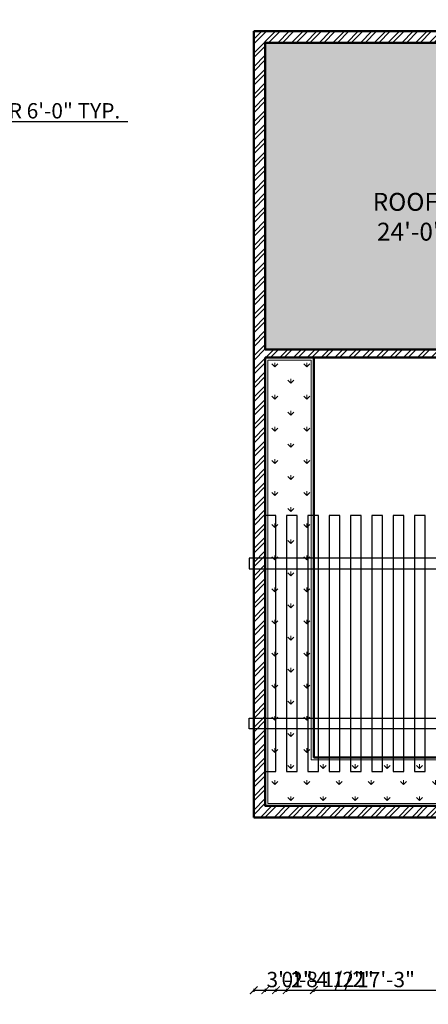
# Model space of a CAD drawing. Units: inches. Extents: x 261 to 2725, y 291 to 1454.
# Tile 26 of 35: x 1824 to 2144, y 293 to 1064. Entities that reach past the tile are written whole.
import ezdxf

# ---------------------------------------------------------------- set-up
doc = ezdxf.new("R2010")
doc.units = ezdxf.units.IN
for name, color, linetype, lineweight in [('A-ANNO-DIMS', 136, 'Continuous', 18), ('A-AREA-IDEN', 18, 'Continuous', 18), ('A-PLNT', 3, 'Continuous', 18), ('A-PLNT-PATT', 3, 'Continuous', 13), ('A-ROOF-PRGL', 25, 'Continuous', 25), ('A-WALL', 222, 'Continuous', 50), ('A-WALL-PATT', 243, 'Continuous', 13)]:
    doc.layers.add(name, color=color, linetype=linetype, lineweight=lineweight)
doc.styles.get("Standard").update_dxf_attribs({"font": 'arial.ttf'})
doc.dimstyles.new('ISO-25', dxfattribs={"dimtxt": 12, "dimasz": 6, "dimexe": 1.25, "dimexo": 0.625, "dimtad": 1, "dimdec": 0, "dimlunit": 3, "dimtxsty": 'Standard', "dimblk": 'ARCHTICK', "dimcen": 2.5, "dimadec": 0, "dimazin": 0, "dimtfac": 1, "dimtdec": 0, "dimtmove": 0, "dimatfit": 3, "dimfxl": 1, "dimfxlon": 1, "dimarcsym": 0})

# ---------------------------------------------------------------- blocks, each defined once
blk = doc.blocks.new('_ArchTick')
at = {"color": 0, "linetype": 'ByBlock', "const_width": 0.15}
blk.add_lwpolyline([(-0.5, -0.5), (0.5, 0.5)], dxfattribs=at)
blk = doc.blocks.new('*D63')
at = {"layer": 'A-ANNO-DIMS', "color": 0, "lineweight": -2, "ltscale": 0.07, "transparency": 16777216}
for p, q in [((1630.08, 983.27), (1630.08, 985.52)), ((1630.08, 984.27), (1702.08, 984.27)), ((1702.08, 983.27), (1702.08, 985.52)), ((1702.08, 984.27), (1909.1, 984.27))]:
    blk.add_line(p, q, dxfattribs=at)
at = {"layer": 'Defpoints', "color": 0, "ltscale": 0.07, "transparency": 16777216}
for p in [(1702.08, 984.27), (1630.08, 973.47), (1702.08, 973.47)]:
    blk.add_point(p, dxfattribs=at)
at = {"layer": 'A-ANNO-DIMS', "color": 0, "lineweight": -2, "ltscale": 0.07, "transparency": 16777216, "xscale": 6, "yscale": 6, "zscale": 6, "rotation": 180}
blk.add_blockref('_ArchTick', (1630.08, 984.27), dxfattribs=at)
at = {"layer": 'A-ANNO-DIMS', "color": 0, "lineweight": -2, "ltscale": 0.07, "transparency": 16777216, "xscale": 6, "yscale": 6, "zscale": 6}
blk.add_blockref('_ArchTick', (1702.08, 984.27), dxfattribs=at)
at = {"layer": 'A-ANNO-DIMS', "color": 0, "ltscale": 0.07, "transparency": 16777216, "insert": (1808.59, 991.1), "char_height": 12, "attachment_point": 5}
blk.add_mtext('SLIDING DOOR 6\'-0" TYP.', dxfattribs=at)
blk = doc.blocks.new('*D82')
at = {"layer": 'A-ANNO-DIMS', "color": 0, "lineweight": -2, "ltscale": 0.07, "transparency": 16777216}
for p, q in [((2600.96, 679.47), (2603.21, 679.47)), ((2601.96, 517.47), (2601.96, 679.47)), ((2600.96, 517.47), (2603.21, 517.47))]:
    blk.add_line(p, q, dxfattribs=at)
at = {"layer": 'Defpoints', "color": 0, "ltscale": 0.07, "transparency": 16777216}
for p in [(946.45, 679.47), (2601.96, 679.47), (946.45, 517.47)]:
    blk.add_point(p, dxfattribs=at)
at = {"layer": 'A-ANNO-DIMS', "color": 0, "lineweight": -2, "ltscale": 0.07, "transparency": 16777216, "xscale": 6, "yscale": 6, "zscale": 6}
for p, rotation in [((2601.96, 679.47), 90), ((2601.96, 517.47), 270)]:
    blk.add_blockref('_ArchTick', p, dxfattribs=dict(at, rotation=rotation))
at = {"layer": 'A-ANNO-DIMS', "color": 0, "ltscale": 0.07, "transparency": 16777216, "insert": (2595.2, 598.47), "char_height": 12, "attachment_point": 5, "rotation": 90}
blk.add_mtext('13\'-6"', dxfattribs=at)
blk = doc.blocks.new('*D83')
at = {"layer": 'A-ANNO-DIMS', "color": 0, "lineweight": -2, "ltscale": 0.07, "transparency": 16777216}
for p, q in [((2600.96, 799.47), (2603.21, 799.47)), ((2601.96, 679.47), (2601.96, 799.47)), ((2600.96, 679.47), (2603.21, 679.47))]:
    blk.add_line(p, q, dxfattribs=at)
at = {"layer": 'Defpoints', "color": 0, "ltscale": 0.07, "transparency": 16777216}
for p in [(946.45, 799.47), (2601.96, 799.47), (946.45, 679.47)]:
    blk.add_point(p, dxfattribs=at)
at = {"layer": 'A-ANNO-DIMS', "color": 0, "lineweight": -2, "ltscale": 0.07, "transparency": 16777216, "xscale": 6, "yscale": 6, "zscale": 6}
for p, rotation in [((2601.96, 799.47), 90), ((2601.96, 679.47), 270)]:
    blk.add_blockref('_ArchTick', p, dxfattribs=dict(at, rotation=rotation))
at = {"layer": 'A-ANNO-DIMS', "color": 0, "ltscale": 0.07, "transparency": 16777216, "insert": (2595.21, 739.47), "char_height": 12, "attachment_point": 5, "rotation": 90}
blk.add_mtext('10\'-0"', dxfattribs=at)
blk = doc.blocks.new('*D84')
at = {"layer": 'A-ANNO-DIMS', "color": 0, "lineweight": -2, "ltscale": 0.07, "transparency": 16777216}
for p, q in [((2600.96, 1024.47), (2603.21, 1024.47)), ((2601.96, 799.47), (2601.96, 1024.47)), ((2600.96, 799.47), (2603.21, 799.47))]:
    blk.add_line(p, q, dxfattribs=at)
at = {"layer": 'Defpoints', "color": 0, "ltscale": 0.07, "transparency": 16777216}
for p in [(946.45, 1024.47), (2601.96, 1024.47), (946.45, 799.47)]:
    blk.add_point(p, dxfattribs=at)
at = {"layer": 'A-ANNO-DIMS', "color": 0, "lineweight": -2, "ltscale": 0.07, "transparency": 16777216, "xscale": 6, "yscale": 6, "zscale": 6}
for p, rotation in [((2601.96, 1024.47), 90), ((2601.96, 799.47), 270)]:
    blk.add_blockref('_ArchTick', p, dxfattribs=dict(at, rotation=rotation))
at = {"layer": 'A-ANNO-DIMS', "color": 0, "ltscale": 0.07, "transparency": 16777216, "insert": (2595.21, 911.97), "char_height": 12, "attachment_point": 5, "rotation": 90}
blk.add_mtext('18\'-9"', dxfattribs=at)
blk = doc.blocks.new('*D85')
at = {"layer": 'A-ANNO-DIMS', "color": 0, "lineweight": -2, "ltscale": 0.07, "transparency": 16777216}
for p, q in [((2600.96, 1222.47), (2603.21, 1222.47)), ((2601.96, 1024.47), (2601.96, 1222.47)), ((2600.96, 1024.47), (2603.21, 1024.47))]:
    blk.add_line(p, q, dxfattribs=at)
at = {"layer": 'Defpoints', "color": 0, "ltscale": 0.07, "transparency": 16777216}
for p in [(946.45, 1222.47), (2601.96, 1222.47), (946.45, 1024.47)]:
    blk.add_point(p, dxfattribs=at)
at = {"layer": 'A-ANNO-DIMS', "color": 0, "lineweight": -2, "ltscale": 0.07, "transparency": 16777216, "xscale": 6, "yscale": 6, "zscale": 6}
for p, rotation in [((2601.96, 1222.47), 90), ((2601.96, 1024.47), 270)]:
    blk.add_blockref('_ArchTick', p, dxfattribs=dict(at, rotation=rotation))
at = {"layer": 'A-ANNO-DIMS', "color": 0, "ltscale": 0.07, "transparency": 16777216, "insert": (2595.21, 1123.47), "char_height": 12, "attachment_point": 5, "rotation": 90}
blk.add_mtext('16\'-6"', dxfattribs=at)
blk = doc.blocks.new('*D89')
at = {"layer": 'A-ANNO-DIMS', "color": 0, "lineweight": -2, "ltscale": 0.07, "transparency": 16777216}
for p, q in [((2600.96, 508.47), (2603.21, 508.47)), ((2601.96, 412.47), (2601.96, 508.47)), ((2600.96, 412.47), (2603.21, 412.47))]:
    blk.add_line(p, q, dxfattribs=at)
at = {"layer": 'Defpoints', "color": 0, "ltscale": 0.07, "transparency": 16777216}
for p in [(955.45, 508.47), (2601.96, 508.47), (994.45, 412.47)]:
    blk.add_point(p, dxfattribs=at)
at = {"layer": 'A-ANNO-DIMS', "color": 0, "lineweight": -2, "ltscale": 0.07, "transparency": 16777216, "xscale": 6, "yscale": 6, "zscale": 6}
for p, rotation in [((2601.96, 508.47), 90), ((2601.96, 412.47), 270)]:
    blk.add_blockref('_ArchTick', p, dxfattribs=dict(at, rotation=rotation))
at = {"layer": 'A-ANNO-DIMS', "color": 0, "ltscale": 0.07, "transparency": 16777216, "insert": (2595.21, 460.47), "char_height": 12, "attachment_point": 5, "rotation": 90}
blk.add_mtext('8\'-0"', dxfattribs=at)
blk = doc.blocks.new('*D111')
at = {"layer": 'A-ANNO-DIMS', "color": 0, "lineweight": -2, "ltscale": 0.07, "transparency": 16777216}
for p, q in [((2600.96, 550.47), (2603.21, 550.47)), ((2601.96, 448.47), (2601.96, 550.47)), ((2600.96, 448.47), (2603.21, 448.47))]:
    blk.add_line(p, q, dxfattribs=at)
at = {"layer": 'Defpoints', "color": 0, "ltscale": 0.07, "transparency": 16777216}
for p in [(1720.08, 550.47), (2601.96, 550.47), (1720.08, 448.47)]:
    blk.add_point(p, dxfattribs=at)
at = {"layer": 'A-ANNO-DIMS', "color": 0, "lineweight": -2, "ltscale": 0.07, "transparency": 16777216, "xscale": 6, "yscale": 6, "zscale": 6}
for p, rotation in [((2601.96, 550.47), 90), ((2601.96, 448.47), 270)]:
    blk.add_blockref('_ArchTick', p, dxfattribs=dict(at, rotation=rotation))
at = {"layer": 'A-ANNO-DIMS', "color": 0, "ltscale": 0.07, "transparency": 16777216, "insert": (2595.21, 499.47), "char_height": 12, "attachment_point": 5, "rotation": 90}
blk.add_mtext('8\'-6"', dxfattribs=at)
blk = doc.blocks.new('*D112')
at = {"layer": 'A-ANNO-DIMS', "color": 0, "lineweight": -2, "ltscale": 0.07, "transparency": 16777216}
for p, q in [((2600.96, 679.47), (2603.21, 679.47)), ((2601.96, 550.47), (2601.96, 679.47)), ((2600.96, 550.47), (2603.21, 550.47))]:
    blk.add_line(p, q, dxfattribs=at)
at = {"layer": 'Defpoints', "color": 0, "ltscale": 0.07, "transparency": 16777216}
for p in [(1720.08, 679.47), (2601.96, 679.47), (1720.08, 550.47)]:
    blk.add_point(p, dxfattribs=at)
at = {"layer": 'A-ANNO-DIMS', "color": 0, "lineweight": -2, "ltscale": 0.07, "transparency": 16777216, "xscale": 6, "yscale": 6, "zscale": 6}
for p, rotation in [((2601.96, 679.47), 90), ((2601.96, 550.47), 270)]:
    blk.add_blockref('_ArchTick', p, dxfattribs=dict(at, rotation=rotation))
at = {"layer": 'A-ANNO-DIMS', "color": 0, "ltscale": 0.07, "transparency": 16777216, "insert": (2595.21, 614.97), "char_height": 12, "attachment_point": 5, "rotation": 90}
blk.add_mtext('10\'-9"', dxfattribs=at)
blk = doc.blocks.new('*D113')
at = {"layer": 'A-ANNO-DIMS', "color": 0, "lineweight": -2, "ltscale": 0.07, "transparency": 16777216}
for p, q in [((2600.96, 799.47), (2603.21, 799.47)), ((2601.96, 679.47), (2601.96, 799.47)), ((2600.96, 679.47), (2603.21, 679.47))]:
    blk.add_line(p, q, dxfattribs=at)
at = {"layer": 'Defpoints', "color": 0, "ltscale": 0.07, "transparency": 16777216}
for p in [(1720.08, 799.47), (2601.96, 799.47), (1720.08, 679.47)]:
    blk.add_point(p, dxfattribs=at)
at = {"layer": 'A-ANNO-DIMS', "color": 0, "lineweight": -2, "ltscale": 0.07, "transparency": 16777216, "xscale": 6, "yscale": 6, "zscale": 6}
for p, rotation in [((2601.96, 799.47), 90), ((2601.96, 679.47), 270)]:
    blk.add_blockref('_ArchTick', p, dxfattribs=dict(at, rotation=rotation))
at = {"layer": 'A-ANNO-DIMS', "color": 0, "ltscale": 0.07, "transparency": 16777216, "insert": (2595.21, 739.47), "char_height": 12, "attachment_point": 5, "rotation": 90}
blk.add_mtext('10\'-0"', dxfattribs=at)
blk = doc.blocks.new('*D114')
at = {"layer": 'A-ANNO-DIMS', "color": 0, "lineweight": -2, "ltscale": 0.07, "transparency": 16777216}
for p, q in [((2600.96, 964.47), (2603.21, 964.47)), ((2601.96, 799.47), (2601.96, 964.47)), ((2600.96, 799.47), (2603.21, 799.47))]:
    blk.add_line(p, q, dxfattribs=at)
at = {"layer": 'Defpoints', "color": 0, "ltscale": 0.07, "transparency": 16777216}
for p in [(1720.08, 964.47), (2601.96, 964.47), (1720.08, 799.47)]:
    blk.add_point(p, dxfattribs=at)
at = {"layer": 'A-ANNO-DIMS', "color": 0, "lineweight": -2, "ltscale": 0.07, "transparency": 16777216, "xscale": 6, "yscale": 6, "zscale": 6}
for p, rotation in [((2601.96, 964.47), 90), ((2601.96, 799.47), 270)]:
    blk.add_blockref('_ArchTick', p, dxfattribs=dict(at, rotation=rotation))
at = {"layer": 'A-ANNO-DIMS', "color": 0, "ltscale": 0.07, "transparency": 16777216, "insert": (2595.2, 881.97), "char_height": 12, "attachment_point": 5, "rotation": 90}
blk.add_mtext('13\'-9"', dxfattribs=at)
blk = doc.blocks.new('*D115')
at = {"layer": 'A-ANNO-DIMS', "color": 0, "lineweight": -2, "ltscale": 0.07, "transparency": 16777216}
for p, q in [((2600.96, 1222.47), (2603.21, 1222.47)), ((2601.96, 964.47), (2601.96, 1222.47)), ((2600.96, 964.47), (2603.21, 964.47))]:
    blk.add_line(p, q, dxfattribs=at)
at = {"layer": 'Defpoints', "color": 0, "ltscale": 0.07, "transparency": 16777216}
for p in [(1720.08, 1222.47), (2601.96, 1222.47), (1720.08, 964.47)]:
    blk.add_point(p, dxfattribs=at)
at = {"layer": 'A-ANNO-DIMS', "color": 0, "lineweight": -2, "ltscale": 0.07, "transparency": 16777216, "xscale": 6, "yscale": 6, "zscale": 6}
for p, rotation in [((2601.96, 1222.47), 90), ((2601.96, 964.47), 270)]:
    blk.add_blockref('_ArchTick', p, dxfattribs=dict(at, rotation=rotation))
at = {"layer": 'A-ANNO-DIMS', "color": 0, "ltscale": 0.07, "transparency": 16777216, "insert": (2595.21, 1093.47), "char_height": 12, "attachment_point": 5, "rotation": 90}
blk.add_mtext('21\'-6"', dxfattribs=at)
blk = doc.blocks.new('*D120')
at = {"layer": 'A-ANNO-DIMS', "color": 0, "lineweight": -2, "ltscale": 0.07, "transparency": 16777216}
for p, q in [((2600.96, 880.73), (2603.21, 880.73)), ((2601.96, 805.47), (2601.96, 880.73)), ((2600.96, 805.47), (2603.21, 805.47))]:
    blk.add_line(p, q, dxfattribs=at)
at = {"layer": 'Defpoints', "color": 0, "ltscale": 0.07, "transparency": 16777216}
for p in [(1559.08, 880.73), (2601.96, 880.73), (1558.08, 805.47)]:
    blk.add_point(p, dxfattribs=at)
at = {"layer": 'A-ANNO-DIMS', "color": 0, "lineweight": -2, "ltscale": 0.07, "transparency": 16777216, "xscale": 6, "yscale": 6, "zscale": 6}
for p, rotation in [((2601.96, 880.73), 90), ((2601.96, 805.47), 270)]:
    blk.add_blockref('_ArchTick', p, dxfattribs=dict(at, rotation=rotation))
at = {"layer": 'A-ANNO-DIMS', "color": 0, "ltscale": 0.07, "transparency": 16777216, "insert": (2595.12, 843.1), "char_height": 12, "attachment_point": 5, "rotation": 90}
blk.add_mtext('6\'-3 1/2"', dxfattribs=at)
blk = doc.blocks.new('*D122')
at = {"layer": 'A-ANNO-DIMS', "color": 0, "lineweight": -2, "ltscale": 0.07, "transparency": 16777216}
for p, q in [((2007.71, 1437.76), (2007.71, 1440.01)), ((2007.71, 1438.76), (2493.71, 1438.76)), ((2493.71, 1437.76), (2493.71, 1440.01))]:
    blk.add_line(p, q, dxfattribs=at)
at = {"layer": 'Defpoints', "color": 0, "ltscale": 0.07, "transparency": 16777216}
for p in [(2493.71, 1438.76), (2007.71, 1054.85), (2493.71, 1054.85)]:
    blk.add_point(p, dxfattribs=at)
at = {"layer": 'A-ANNO-DIMS', "color": 0, "lineweight": -2, "ltscale": 0.07, "transparency": 16777216, "xscale": 6, "yscale": 6, "zscale": 6, "rotation": 180}
blk.add_blockref('_ArchTick', (2007.71, 1438.76), dxfattribs=at)
at = {"layer": 'A-ANNO-DIMS', "color": 0, "lineweight": -2, "ltscale": 0.07, "transparency": 16777216, "xscale": 6, "yscale": 6, "zscale": 6}
blk.add_blockref('_ArchTick', (2493.71, 1438.76), dxfattribs=at)
at = {"layer": 'A-ANNO-DIMS', "color": 0, "ltscale": 0.07, "transparency": 16777216, "insert": (2250.71, 1445.51), "char_height": 12, "attachment_point": 5}
blk.add_mtext('40\'-6"', dxfattribs=at)
blk = doc.blocks.new('*D123')
at = {"layer": 'A-ANNO-DIMS', "color": 0, "lineweight": -2, "ltscale": 0.07, "transparency": 16777216}
for p, q in [((287.06, 1054.85), (284.81, 1054.85)), ((286.06, 439.47), (286.06, 1054.85)), ((287.06, 439.47), (284.81, 439.47))]:
    blk.add_line(p, q, dxfattribs=at)
at = {"layer": 'Defpoints', "color": 0, "ltscale": 0.07, "transparency": 16777216}
for p in [(286.06, 1054.85), (2007.71, 1054.85), (2007.71, 439.47)]:
    blk.add_point(p, dxfattribs=at)
at = {"layer": 'A-ANNO-DIMS', "color": 0, "lineweight": -2, "ltscale": 0.07, "transparency": 16777216, "xscale": 6, "yscale": 6, "zscale": 6}
for p, rotation in [((286.06, 1054.85), 90), ((286.06, 439.47), 270)]:
    blk.add_blockref('_ArchTick', p, dxfattribs=dict(at, rotation=rotation))
at = {"layer": 'A-ANNO-DIMS', "color": 0, "ltscale": 0.07, "transparency": 16777216, "insert": (279.22, 747.16), "char_height": 12, "attachment_point": 5, "rotation": 90}
blk.add_mtext('51\'-3 1/2"', dxfattribs=at)
blk = doc.blocks.new('*D124')
at = {"layer": 'A-ANNO-DIMS', "color": 0, "lineweight": -2, "ltscale": 0.07, "transparency": 16777216}
for p, q in [((2007.71, 305.22), (2007.71, 302.97)), ((2007.71, 304.22), (2214.67, 304.22)), ((2214.67, 305.22), (2214.67, 302.97))]:
    blk.add_line(p, q, dxfattribs=at)
at = {"layer": 'Defpoints', "color": 0, "ltscale": 0.07, "transparency": 16777216}
for p in [(2007.71, 439.47), (2214.67, 439.47), (2214.67, 304.22)]:
    blk.add_point(p, dxfattribs=at)
at = {"layer": 'A-ANNO-DIMS', "color": 0, "lineweight": -2, "ltscale": 0.07, "transparency": 16777216, "xscale": 6, "yscale": 6, "zscale": 6, "rotation": 180}
blk.add_blockref('_ArchTick', (2007.71, 304.22), dxfattribs=at)
at = {"layer": 'A-ANNO-DIMS', "color": 0, "lineweight": -2, "ltscale": 0.07, "transparency": 16777216, "xscale": 6, "yscale": 6, "zscale": 6}
blk.add_blockref('_ArchTick', (2214.67, 304.22), dxfattribs=at)
at = {"layer": 'A-ANNO-DIMS', "color": 0, "ltscale": 0.07, "transparency": 16777216, "insert": (2111.19, 310.97), "char_height": 12, "attachment_point": 5}
blk.add_mtext('17\'-3"', dxfattribs=at)
blk = doc.blocks.new('*D129')
at = {"layer": 'A-ANNO-DIMS', "color": 0, "lineweight": -2, "ltscale": 0.07, "transparency": 16777216}
for p, q in [((2016.71, 305.22), (2016.71, 302.97)), ((2016.71, 304.22), (2054.71, 304.22)), ((2054.71, 305.22), (2054.71, 302.97))]:
    blk.add_line(p, q, dxfattribs=at)
at = {"layer": 'Defpoints', "color": 0, "ltscale": 0.07, "transparency": 16777216}
for p in [(2016.71, 799.47), (2054.71, 799.47), (2054.71, 304.22)]:
    blk.add_point(p, dxfattribs=at)
at = {"layer": 'A-ANNO-DIMS', "color": 0, "lineweight": -2, "ltscale": 0.07, "transparency": 16777216, "xscale": 6, "yscale": 6, "zscale": 6, "rotation": 180}
blk.add_blockref('_ArchTick', (2016.71, 304.22), dxfattribs=at)
at = {"layer": 'A-ANNO-DIMS', "color": 0, "lineweight": -2, "ltscale": 0.07, "transparency": 16777216, "xscale": 6, "yscale": 6, "zscale": 6}
blk.add_blockref('_ArchTick', (2054.71, 304.22), dxfattribs=at)
at = {"layer": 'A-ANNO-DIMS', "color": 0, "ltscale": 0.07, "transparency": 16777216, "insert": (2035.71, 310.97), "char_height": 12, "attachment_point": 5}
blk.add_mtext('3\'-2"', dxfattribs=at)
blk = doc.blocks.new('*D133')
at = {"layer": 'A-ANNO-DIMS', "color": 0, "lineweight": -2, "ltscale": 0.07, "transparency": 16777216}
for p, q in [((2016.71, 305.22), (2016.71, 302.97)), ((2016.71, 304.22), (2025.05, 304.22)), ((2025.05, 305.22), (2025.05, 302.97)), ((2025.05, 304.22), (2092.16, 304.22))]:
    blk.add_line(p, q, dxfattribs=at)
at = {"layer": 'Defpoints', "color": 0, "ltscale": 0.07, "transparency": 16777216}
for p in [(2016.71, 675.78), (2025.05, 675.78), (2025.05, 304.22)]:
    blk.add_point(p, dxfattribs=at)
at = {"layer": 'A-ANNO-DIMS', "color": 0, "lineweight": -2, "ltscale": 0.07, "transparency": 16777216, "xscale": 6, "yscale": 6, "zscale": 6, "rotation": 180}
blk.add_blockref('_ArchTick', (2016.71, 304.22), dxfattribs=at)
at = {"layer": 'A-ANNO-DIMS', "color": 0, "lineweight": -2, "ltscale": 0.07, "transparency": 16777216, "xscale": 6, "yscale": 6, "zscale": 6}
blk.add_blockref('_ArchTick', (2025.05, 304.22), dxfattribs=at)
at = {"layer": 'A-ANNO-DIMS', "color": 0, "ltscale": 0.07, "transparency": 16777216, "insert": (2061.61, 311.05), "char_height": 12, "attachment_point": 5}
blk.add_mtext('0\'-8 1/2"', dxfattribs=at)
blk = doc.blocks.new('*D134')
at = {"layer": 'A-ANNO-DIMS', "color": 0, "lineweight": -2, "ltscale": 0.07, "transparency": 16777216}
for p, q in [((2016.71, 305.22), (2016.71, 302.97)), ((2016.71, 304.22), (2033.4, 304.22)), ((2033.4, 305.22), (2033.4, 302.97)), ((2033.4, 304.22), (2099.38, 304.22))]:
    blk.add_line(p, q, dxfattribs=at)
at = {"layer": 'Defpoints', "color": 0, "ltscale": 0.07, "transparency": 16777216}
for p in [(2016.71, 475.47), (2033.4, 475.47), (2033.4, 304.22)]:
    blk.add_point(p, dxfattribs=at)
at = {"layer": 'A-ANNO-DIMS', "color": 0, "lineweight": -2, "ltscale": 0.07, "transparency": 16777216, "xscale": 6, "yscale": 6, "zscale": 6, "rotation": 180}
blk.add_blockref('_ArchTick', (2016.71, 304.22), dxfattribs=at)
at = {"layer": 'A-ANNO-DIMS', "color": 0, "lineweight": -2, "ltscale": 0.07, "transparency": 16777216, "xscale": 6, "yscale": 6, "zscale": 6}
blk.add_blockref('_ArchTick', (2033.4, 304.22), dxfattribs=at)
at = {"layer": 'A-ANNO-DIMS', "color": 0, "ltscale": 0.07, "transparency": 16777216, "insert": (2069.39, 311.05), "char_height": 12, "attachment_point": 5}
blk.add_mtext('1\'-4 1/2"', dxfattribs=at)
blk = doc.blocks.new('*D135')
at = {"layer": 'A-ANNO-DIMS', "color": 0, "lineweight": -2, "ltscale": 0.07, "transparency": 16777216}
for p, q in [((2004.19, 1437.76), (2004.19, 1440.01)), ((2004.19, 1438.76), (2221.19, 1438.76)), ((2221.19, 1437.76), (2221.19, 1440.01))]:
    blk.add_line(p, q, dxfattribs=at)
at = {"layer": 'Defpoints', "color": 0, "ltscale": 0.07, "transparency": 16777216}
for p in [(2221.19, 1438.76), (2004.19, 642.39), (2221.19, 642.39)]:
    blk.add_point(p, dxfattribs=at)
at = {"layer": 'A-ANNO-DIMS', "color": 0, "lineweight": -2, "ltscale": 0.07, "transparency": 16777216, "xscale": 6, "yscale": 6, "zscale": 6, "rotation": 180}
blk.add_blockref('_ArchTick', (2004.19, 1438.76), dxfattribs=at)
at = {"layer": 'A-ANNO-DIMS', "color": 0, "lineweight": -2, "ltscale": 0.07, "transparency": 16777216, "xscale": 6, "yscale": 6, "zscale": 6}
blk.add_blockref('_ArchTick', (2221.19, 1438.76), dxfattribs=at)
at = {"layer": 'A-ANNO-DIMS', "color": 0, "ltscale": 0.07, "transparency": 16777216, "insert": (2112.69, 1445.51), "char_height": 12, "attachment_point": 5}
blk.add_mtext('18\'-1"', dxfattribs=at)

msp = doc.modelspace()

# ---------------------------------------------------------------- hatches: boundary and pattern name
at = {"layer": 'A-PLNT-PATT'}
h = msp.add_hatch(dxfattribs=at)
h.set_pattern_fill('GRASS', color=256, scale=0.7)
h.paths.add_polyline_path([(658.45, 427.47), (433.45, 427.47), (433.45, 415.47), (658.45, 415.47)])
h.paths.add_polyline_path([(670.45, 421.47), (664.45, 421.47), (664.45, 415.47), (670.45, 415.47)])
h.paths.add_polyline_path([(784.45, 421.47), (778.45, 421.47), (778.45, 415.47), (784.45, 415.47)])
h.paths.add_polyline_path([(991.45, 427.47), (790.45, 427.47), (790.45, 415.47), (991.45, 415.47)])
h.paths.add_polyline_path([(1439.08, 1220.47), (1252.08, 1220.47), (1252.08, 1198.47), (1417.08, 1198.47), (1417.08, 1117.47), (1439.08, 1117.47)])
h.paths.add_polyline_path([(2304.71, 1045.85), (2016.71, 1045.85), (2016.71, 805.87), (2304.71, 805.87)])
h.paths.add_polyline_path([(1267.21, 1201.68), (1431.59, 1201.68), (1431.59, 1218.76), (1267.21, 1218.76)], flags=24)
h.paths.add_polyline_path([(2089.2, 883.04), (2242.64, 883.04), (2242.64, 936.27), (2089.2, 936.27)], flags=24)
h = msp.add_hatch(dxfattribs=at)
h.set_pattern_fill('GRASS', color=256, scale=0.7)
h.paths.add_polyline_path([(2052.71, 797.47), (2018.71, 797.47), (2018.71, 450.47), (2206.67, 450.47), (2206.67, 507.47), (2482.71, 507.47), (2482.71, 671.47), (2448.71, 671.47), (2448.71, 541.47), (2172.67, 541.47), (2172.67, 484.47), (2052.71, 484.47)])
at = {"layer": 'A-WALL-PATT'}
h = msp.add_hatch(dxfattribs=at)
h.set_pattern_fill('ANSI32', color=256, scale=0.8)
h.paths.add_polyline_path([(478.45, 685.47), (580.45, 685.47), (580.45, 691.47), (577.45, 691.47), (577.45, 694.47), (571.45, 694.47), (571.45, 691.47), (478.45, 691.47), (478.45, 721.47), (469.45, 721.47), (469.45, 508.47), (538.45, 508.47), (538.45, 517.47), (478.45, 517.47)])
h.paths.add_polyline_path([(694.45, 517.47), (676.45, 517.47), (676.45, 646.47), (670.45, 646.47), (670.45, 517.47), (610.45, 517.47), (610.45, 508.47), (694.45, 508.47)])
h.paths.add_polyline_path([(676.45, 784.47), (478.45, 784.47), (478.45, 844.47), (469.45, 844.47), (469.45, 745.47), (478.45, 745.47), (478.45, 775.47), (571.45, 775.47), (571.45, 724.47), (577.45, 724.47), (577.45, 775.47), (670.45, 775.47), (670.45, 691.47), (610.45, 691.47), (610.45, 685.47), (670.45, 685.47), (670.45, 682.47), (676.45, 682.47)])
h.paths.add_polyline_path([(955.45, 880.47), (946.45, 880.47), (946.45, 808.47), (778.45, 808.47), (778.45, 799.47), (946.45, 799.47), (946.45, 517.47), (898.45, 517.47), (898.45, 508.47), (955.45, 508.47)])
h.paths.add_polyline_path([(778.45, 598.47), (772.45, 598.47), (772.45, 517.47), (754.45, 517.47), (754.45, 508.47), (826.45, 508.47), (826.45, 517.47), (778.45, 517.47)])
h.paths.add_polyline_path([(955.45, 1090.47), (946.45, 1090.47), (946.45, 1030.47), (817.45, 1030.47), (817.45, 1024.47), (946.45, 1024.47), (946.45, 952.47), (955.45, 952.47)])
h.paths.add_polyline_path([(955.45, 1231.47), (730.45, 1231.47), (730.45, 1222.47), (772.45, 1222.47), (772.45, 1096.47), (766.45, 1096.47), (766.45, 1090.47), (772.45, 1090.47), (772.45, 1006.47), (712.45, 1006.47), (712.45, 1000.47), (778.45, 1000.47), (778.45, 1024.47), (781.45, 1024.47), (781.45, 1030.47), (778.45, 1030.47), (778.45, 1222.47), (946.45, 1222.47), (946.45, 1162.47), (955.45, 1162.47)])
h.paths.add_polyline_path([(694.45, 1231.47), (619.45, 1231.47), (619.45, 1222.47), (646.45, 1222.47), (646.45, 1039.47), (652.45, 1039.47), (652.45, 1090.47), (736.45, 1090.47), (736.45, 1096.47), (652.45, 1096.47), (652.45, 1222.47), (694.45, 1222.47)])
h.paths.add_polyline_path([(571.45, 1231.47), (469.45, 1231.47), (469.45, 1099.47), (478.45, 1099.47), (478.45, 1144.47), (544.45, 1144.47), (544.45, 1153.47), (538.45, 1153.47), (538.45, 1150.47), (478.45, 1150.47), (478.45, 1222.47), (538.45, 1222.47), (538.45, 1183.47), (544.45, 1183.47), (544.45, 1222.47), (571.45, 1222.47)])
h.paths.add_polyline_path([(538.45, 1006.47), (478.45, 1006.47), (478.45, 1051.47), (469.45, 1051.47), (469.45, 940.47), (478.45, 940.47), (478.45, 1000.47), (538.45, 1000.47)])
h.paths.add_polyline_path([(652.45, 1006.47), (652.45, 1009.47), (646.45, 1009.47), (646.45, 1006.47), (586.45, 1006.47), (586.45, 1000.47), (652.45, 1000.47)])
h.paths.add_polyline_path([(1288.08, 973.47), (1243.08, 973.47), (1243.08, 920.97), (1252.08, 920.97), (1252.08, 964.47), (1288.08, 964.47)], flags=17)
h.paths.add_polyline_path([(1402.08, 805.47), (1252.08, 805.47), (1252.08, 848.97), (1243.08, 848.97), (1243.08, 757.47), (1252.08, 757.47), (1252.08, 799.47), (1294.08, 799.47), (1372.08, 799.47), (1372.08, 779.47), (1372.08, 715.47), (1378.08, 715.47), (1378.08, 799.47), (1402.08, 799.47)])
h.paths.add_polyline_path([(1252.08, 721.47), (1243.08, 721.47), (1243.08, 439.47), (1729.08, 439.47), (1729.08, 709.47), (1720.08, 709.47), (1720.08, 679.47), (1582.08, 679.47), (1582.08, 670.47), (1588.08, 670.47), (1588.08, 673.47), (1720.08, 673.47), (1720.08, 559.47), (1690.08, 559.47), (1690.08, 550.47), (1720.08, 550.47), (1720.08, 448.47), (1252.08, 448.47), (1252.08, 496.47), (1312.08, 496.47), (1312.08, 505.47), (1252.08, 505.47), (1252.08, 673.47), (1405.08, 673.47), (1405.08, 679.47), (1378.08, 679.47), (1378.08, 685.47), (1372.08, 685.47), (1372.08, 679.47), (1252.08, 679.47)])
h.paths.add_polyline_path([(1450.08, 550.47), (1480.08, 550.47), (1480.08, 559.47), (1450.08, 559.47), (1450.08, 679.47), (1441.08, 679.47), (1441.08, 673.47), (1444.08, 673.47), (1444.08, 505.47), (1384.08, 505.47), (1384.08, 496.47), (1450.08, 496.47)], flags=17)
h.paths.add_polyline_path([(1618.08, 559.47), (1588.08, 559.47), (1588.08, 634.47), (1582.08, 634.47), (1582.08, 559.47), (1552.08, 559.47), (1552.08, 550.47), (1618.08, 550.47)], flags=17)
h.paths.add_polyline_path([(1564.08, 964.47), (1630.08, 964.47), (1630.08, 973.47), (1477.08, 973.47), (1477.08, 964.47), (1558.08, 964.47), (1558.08, 926.22), (1558.08, 887.97), (1486.08, 887.97), (1486.08, 881.97), (1558.08, 881.97), (1558.08, 805.47), (1450.08, 805.47), (1450.08, 845.97), (1444.08, 845.97), (1444.08, 805.47), (1438.08, 805.47), (1438.08, 799.47), (1564.08, 799.47)], flags=17)
h.paths.add_polyline_path([(1453.08, 973.47), (1408.08, 973.47), (1408.08, 964.47), (1444.08, 964.47), (1444.08, 881.97), (1450.08, 881.97), (1456.08, 881.97), (1456.08, 887.97), (1450.08, 887.97), (1450.08, 964.47), (1453.08, 964.47)], flags=17)
h.paths.add_polyline_path([(1729.08, 1231.47), (1243.08, 1231.47), (1243.08, 1167.47), (1252.08, 1167.47), (1252.08, 1222.47), (1441.08, 1222.47), (1441.08, 1045.47), (1648.08, 1045.47), (1648.08, 1051.47), (1450.08, 1051.47), (1450.08, 1074.47), (1450.08, 1222.47), (1472.08, 1222.47), (1720.08, 1222.47), (1720.08, 1051.47), (1708.08, 1051.47), (1708.08, 1045.47), (1720.08, 1045.47), (1720.08, 973.47), (1702.08, 973.47), (1702.08, 964.47), (1720.08, 964.47), (1720.08, 769.47), (1729.08, 769.47)])
h.paths.add_polyline_path([(2493.71, 1054.85), (2007.71, 1054.85), (2007.71, 439.47), (2214.67, 439.47), (2214.67, 496.47), (2493.71, 496.47)])
h.paths.add_polyline_path([(2016.71, 1045.85), (2304.71, 1045.85), (2304.71, 841.47), (2310.71, 841.47), (2310.71, 1045.85), (2484.71, 1045.85), (2484.71, 805.47), (2310.71, 805.47), (2310.71, 811.47), (2304.71, 811.47), (2304.71, 799.47), (2484.71, 799.47), (2484.71, 679.47), (2304.71, 679.47), (2304.71, 673.47), (2484.71, 673.47), (2484.71, 505.47), (2208.67, 505.47), (2208.67, 448.47), (2016.71, 448.47), (2016.71, 799.47), (2304.71, 799.47), (2304.71, 805.47), (2016.71, 805.47)], flags=16)

# ---------------------------------------------------------------- linework, layer by layer
at = {"layer": 'A-PLNT'}
msp.add_line((2018.71, 797.47), (2052.71, 797.47), dxfattribs=at)
msp.add_lwpolyline([(2016.71, 1045.85), (2304.71, 1045.85), (2304.71, 805.87), (2016.71, 805.87)], close=True, dxfattribs=at)
for points in [[(2018.71, 797.47), (2018.71, 450.47), (2206.67, 450.47), (2206.67, 507.47), (2482.71, 507.47), (2482.71, 671.47)], [(2052.71, 797.47), (2052.71, 484.47), (2172.67, 484.47), (2172.67, 541.47), (2448.71, 541.47), (2448.71, 671.47)]]:
    msp.add_lwpolyline(points, dxfattribs=at)
at = {"layer": 'A-ROOF-PRGL'}
for points in [[(2016.71, 475.47), (2025.05, 475.47), (2025.05, 675.78), (2016.71, 675.78)], [(2033.4, 475.47), (2041.75, 475.47), (2041.75, 675.78), (2033.4, 675.78)], [(2050.09, 475.47), (2058.44, 475.47), (2058.44, 675.78), (2050.09, 675.78)], [(2066.79, 475.47), (2075.13, 475.47), (2075.13, 675.78), (2066.79, 675.78)], [(2083.48, 475.47), (2091.82, 475.47), (2091.82, 675.78), (2083.48, 675.78)], [(2100.17, 475.47), (2108.52, 475.47), (2108.52, 675.78), (2100.17, 675.78)], [(2116.86, 475.47), (2125.21, 475.47), (2125.21, 675.78), (2116.86, 675.78)], [(2133.56, 475.47), (2141.9, 475.47), (2141.9, 675.78), (2133.56, 675.78)], [(2004.19, 634.05), (2221.19, 634.05), (2221.19, 642.39), (2004.19, 642.39)], [(2004.19, 517.2), (2221.19, 517.2), (2221.19, 508.85), (2004.19, 508.85)]]:
    msp.add_lwpolyline(points, close=True, dxfattribs=at)
at = {"layer": 'A-WALL'}
for p, q in [((2007.71, 439.47), (2007.71, 1054.85)), ((2007.71, 1054.85), (2493.71, 1054.85)), ((2016.71, 1045.85), (2304.71, 1045.85)), ((2016.71, 1045.85), (2016.71, 805.87)), ((2016.71, 805.87), (2304.71, 805.87)), ((2016.71, 799.47), (2484.71, 799.47)), ((2007.71, 439.47), (2214.67, 439.47))]:
    msp.add_line(p, q, dxfattribs=at)
for points in [[(2016.71, 799.47), (2016.71, 448.47), (2208.67, 448.47), (2208.67, 505.47), (2484.71, 505.47), (2484.71, 673.47)], [(2054.71, 799.47), (2054.71, 486.47), (2170.67, 486.47), (2170.67, 543.47), (2446.71, 543.47), (2446.71, 673.47)]]:
    msp.add_lwpolyline(points, dxfattribs=at)

# ---------------------------------------------------------------- texts
at = {"layer": 'A-AREA-IDEN', "insert": (2091.71, 928.35), "char_height": 14, "attachment_point": 1}
msp.add_mtext_dynamic_manual_height_columns('\\pxqc;{\\fTimes New Roman|b0|i0|c0|p18;ROOF GARDEN\\P24\'-0" x 20\'-0"}', width=148.4764, gutter_width=12.5, heights=[0], dxfattribs=at)

# ---------------------------------------------------------------- dimensions: what is measured, and where the dimension line sits
at = {"layer": 'A-ANNO-DIMS', "ltscale": 0.07}
for base, p1, p2, picture, middle in [((2221.19, 1438.76), (2004.19, 642.39), (2221.19, 642.39), '*D135', (2112.69, 1445.51)), ((2493.71, 1438.76), (2007.71, 1054.85), (2493.71, 1054.85), '*D122', (2250.71, 1445.51)), ((2054.71, 304.22), (2016.71, 799.47), (2054.71, 799.47), '*D129', (2035.71, 310.97)), ((2025.05, 304.22), (2016.71, 675.78), (2025.05, 675.78), '*D133', (2061.61, 311.05)), ((2033.4, 304.22), (2016.71, 475.47), (2033.4, 475.47), '*D134', (2069.39, 311.05)), ((2214.67, 304.22), (2007.71, 439.47), (2214.67, 439.47), '*D124', (2111.19, 310.97))]:
    dim = msp.add_linear_dim(base=base, p1=p1, p2=p2, dimstyle='ISO-25', override={"dimdec": 1, "dimlfac": 1, "dimrnd": 0, "dimzin": 1, "dimdsep": 46, "dimlunit": 4, "dimfrac": 2}, dxfattribs=at)
    dim.commit()
    dim.dimension.update_dxf_attribs({"geometry": picture, "text_midpoint": middle})
for base, p1, p2, picture, middle in [((2601.96, 1222.47), (946.45, 1024.47), (946.45, 1222.47), '*D85', (2595.21, 1123.47)), ((2601.96, 1222.47), (1720.08, 964.47), (1720.08, 1222.47), '*D115', (2595.21, 1093.47)), ((286.06, 1054.85), (2007.71, 439.47), (2007.71, 1054.85), '*D123', (279.22, 747.16)), ((2601.96, 1024.47), (946.45, 799.47), (946.45, 1024.47), '*D84', (2595.21, 911.97)), ((2601.96, 964.47), (1720.08, 799.47), (1720.08, 964.47), '*D114', (2595.2, 881.97)), ((2601.96, 880.73), (1558.08, 805.47), (1559.08, 880.73), '*D120', (2595.12, 843.1)), ((2601.96, 799.47), (946.45, 679.47), (946.45, 799.47), '*D83', (2595.21, 739.47)), ((2601.96, 799.47), (1720.08, 679.47), (1720.08, 799.47), '*D113', (2595.21, 739.47)), ((2601.96, 679.47), (946.45, 517.47), (946.45, 679.47), '*D82', (2595.2, 598.47)), ((2601.96, 679.47), (1720.08, 550.47), (1720.08, 679.47), '*D112', (2595.21, 614.97)), ((2601.96, 550.47), (1720.08, 448.47), (1720.08, 550.47), '*D111', (2595.21, 499.47)), ((2601.96, 508.47), (994.45, 412.47), (955.45, 508.47), '*D89', (2595.21, 460.47))]:
    dim = msp.add_linear_dim(base=base, p1=p1, p2=p2, angle=90, dimstyle='ISO-25', override={"dimdec": 1, "dimlfac": 1, "dimrnd": 0, "dimzin": 1, "dimdsep": 46, "dimlunit": 4, "dimfrac": 2}, dxfattribs=at)
    dim.commit()
    dim.dimension.update_dxf_attribs({"geometry": picture, "text_midpoint": middle})
dim = msp.add_linear_dim(base=(1702.08, 984.27), p1=(1630.08, 973.47), p2=(1702.08, 973.47), text='SLIDING DOOR <> TYP.', dimstyle='ISO-25', override={"dimdec": 1, "dimrnd": 0, "dimzin": 1, "dimlunit": 4, "dimfrac": 2}, dxfattribs=at)
dim.commit()
dim.dimension.update_dxf_attribs({"geometry": '*D63', "text_midpoint": (1808.59, 991.1)})

doc.saveas('drawing.dxf')
